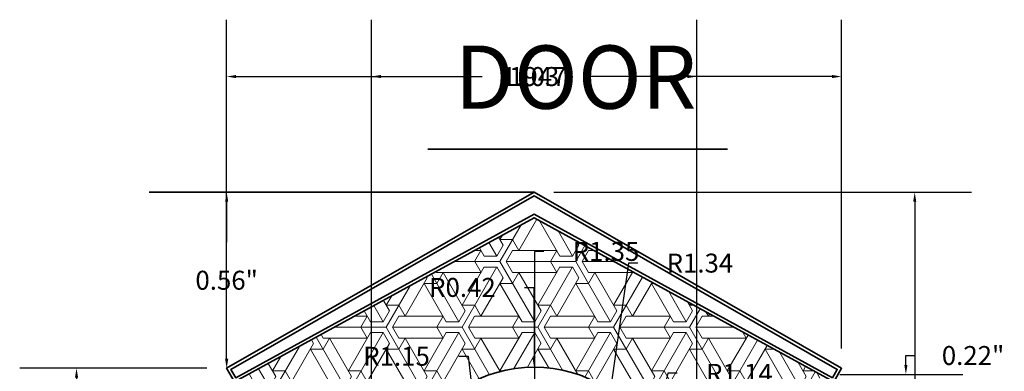
# Model space of a CAD drawing. Units: inches. Extents: x 19.36 to 24.97, y -1.46 to 4.09.
# Tile 4 of 4: x 19.36 to 22.48, y 2.98 to 4.09. Entities that reach past the tile are written whole.
import ezdxf

# ---------------------------------------------------------------- set-up
doc = ezdxf.new("R2010")
doc.units = ezdxf.units.IN
doc.header["$MEASUREMENT"] = 0
for name, color, linetype, lineweight in [('A-ANNO-DIMS', 2, 'Continuous', 18), ('A-ANNO-TEXT', 7, 'Continuous', 25), ('A-ELEV', 7, 'Continuous', 35), ('A-ELEV-PATT', 8, 'Continuous', 13)]:
    doc.layers.add(name, color=color, linetype=linetype, lineweight=lineweight)
doc.styles.get("Standard").update_dxf_attribs({"font": 'arial.ttf'})
doc.dimstyles.get("Standard").update_dxf_attribs({"dimtxt": 0.06, "dimasz": 0.03, "dimexe": 0.18, "dimexo": 0.0625, "dimgap": 0.09, "dimtad": 0, "dimtih": 1, "dimtoh": 1, "dimzin": 0, "dimdsep": 46, "dimlunit": 3, "dimtxsty": 'Standard', "dimcen": 0, "dimadec": 0, "dimazin": 0, "dimtfac": 1, "dimtofl": 0, "dimtmove": 0, "dimatfit": 3, "dimfxl": 1, "dimtolj": 1, "dimtzin": 0, "dimarcsym": 1})

# ---------------------------------------------------------------- blocks, each defined once
blk = doc.blocks.new('*D3')
at = {"layer": 'A-ANNO-DIMS', "color": 0, "lineweight": -2, "transparency": 16777216}
for p, q in [((19.9523, 3.5451), (19.8348, 3.5451)), ((20.0148, 3.5151), (20.0148, 3.3871)), ((20.0148, 3.0177), (20.0148, 3.1458)), ((19.9523, 2.9877), (19.8348, 2.9877))]:
    blk.add_line(p, q, dxfattribs=at)
at = {"layer": 'A-ANNO-DIMS', "color": 0, "transparency": 16777216}
for points in [[(20.0098, 3.5151), (20.0198, 3.5151), (20.0148, 3.5451)], [(20.0098, 3.0177), (20.0198, 3.0177), (20.0148, 2.9877)]]:
    blk.add_solid(points, dxfattribs=at)
at = {"layer": 'Defpoints', "color": 0, "transparency": 16777216}
for p in [(20.0148, 3.5451), (20.0148, 3.5451), (20.0148, 2.9877)]:
    blk.add_point(p, dxfattribs=at)
at = {"layer": 'A-ANNO-DIMS', "color": 0, "transparency": 16777216, "insert": (20.0148, 3.2664), "char_height": 0.06, "width": 0.223205, "attachment_point": 5}
blk.add_mtext('\\A1;0.56"', dxfattribs=at)
blk = doc.blocks.new('*D6')
at = {"layer": 'A-ANNO-DIMS', "color": 0, "lineweight": -2, "transparency": 16777216}
for p, q in [((22.1656, 2.9981), (22.1656, 3.0281)), ((22.1656, 3.0281), (22.1956, 3.0281)), ((21.9561, 2.9681), (22.3456, 2.9681)), ((21.9561, 2.75), (22.3456, 2.75)), ((22.1656, 2.72), (22.1656, 2.69))]:
    blk.add_line(p, q, dxfattribs=at)
at = {"layer": 'A-ANNO-DIMS', "color": 0, "transparency": 16777216}
for points in [[(22.1606, 2.9981), (22.1706, 2.9981), (22.1656, 2.9681)], [(22.1606, 2.72), (22.1706, 2.72), (22.1656, 2.75)]]:
    blk.add_solid(points, dxfattribs=at)
at = {"layer": 'Defpoints', "color": 0, "transparency": 16777216}
for p in [(21.8936, 2.9681), (22.1656, 2.9681), (21.8936, 2.75)]:
    blk.add_point(p, dxfattribs=at)
at = {"layer": 'A-ANNO-DIMS', "color": 0, "transparency": 16777216, "insert": (22.3783, 3.0281), "char_height": 0.06, "attachment_point": 5}
blk.add_mtext('\\A1;0.22"', dxfattribs=at)
blk = doc.blocks.new('*D20')
at = {"layer": 'A-ANNO-DIMS', "color": 0, "lineweight": -2, "transparency": 16777216}
for p, q in [((21.0509, 3.5451), (22.3736, 3.5451)), ((22.1936, 3.5151), (22.1936, 1.9182)), ((22.1936, 0.08), (22.1936, 1.6769)), ((22.0261, 0.05), (22.3736, 0.05))]:
    blk.add_line(p, q, dxfattribs=at)
at = {"layer": 'A-ANNO-DIMS', "color": 0, "transparency": 16777216}
for points in [[(22.1886, 3.5151), (22.1986, 3.5151), (22.1936, 3.5451)], [(22.1886, 0.08), (22.1986, 0.08), (22.1936, 0.05)]]:
    blk.add_solid(points, dxfattribs=at)
at = {"layer": 'Defpoints', "color": 0, "transparency": 16777216}
for p in [(20.9884, 3.5451), (22.1936, 3.5451), (21.9636, 0.05)]:
    blk.add_point(p, dxfattribs=at)
at = {"layer": 'A-ANNO-DIMS', "color": 0, "transparency": 16777216, "insert": (22.1936, 1.7976), "char_height": 0.06, "attachment_point": 5}
blk.add_mtext('\\A1;3.495', dxfattribs=at)
blk = doc.blocks.new('*D21')
at = {"layer": 'A-ANNO-DIMS', "color": 0, "lineweight": -2, "transparency": 16777216}
for p, q in [((20.4736, 0.1125), (20.4736, 4.0914)), ((21.5036, 0.1125), (21.5036, 4.0914)), ((20.5036, 3.9114), (20.8235, 3.9114)), ((21.4736, 3.9114), (21.1537, 3.9114))]:
    blk.add_line(p, q, dxfattribs=at)
at = {"layer": 'A-ANNO-DIMS', "color": 0, "transparency": 16777216}
for points in [[(20.5036, 3.9164), (20.5036, 3.9064), (20.4736, 3.9114)], [(21.4736, 3.9164), (21.4736, 3.9064), (21.5036, 3.9114)]]:
    blk.add_solid(points, dxfattribs=at)
at = {"layer": 'Defpoints', "color": 0, "transparency": 16777216}
for p in [(21.5036, 3.9114), (20.4736, 0.05), (21.5036, 0.05)]:
    blk.add_point(p, dxfattribs=at)
at = {"layer": 'A-ANNO-DIMS', "color": 0, "transparency": 16777216, "insert": (20.9886, 3.9114), "char_height": 0.06, "attachment_point": 5}
blk.add_mtext('\\A1;1.03', dxfattribs=at)
blk = doc.blocks.new('*D27')
at = {"layer": 'A-ANNO-DIMS', "color": 0, "lineweight": -2, "transparency": 16777216}
for p, q in [((19.9523, 2.9877), (19.3594, 2.9877)), ((19.5394, 2.9577), (19.5394, 1.6395)), ((19.5394, 0.08), (19.5394, 1.3982)), ((19.9511, 0.05), (19.3594, 0.05))]:
    blk.add_line(p, q, dxfattribs=at)
at = {"layer": 'A-ANNO-DIMS', "color": 0, "transparency": 16777216}
for points in [[(19.5344, 2.9577), (19.5444, 2.9577), (19.5394, 2.9877)], [(19.5344, 0.08), (19.5444, 0.08), (19.5394, 0.05)]]:
    blk.add_solid(points, dxfattribs=at)
at = {"layer": 'Defpoints', "color": 0, "transparency": 16777216}
for p in [(20.0148, 2.9877), (19.5394, 0.05), (20.0136, 0.05)]:
    blk.add_point(p, dxfattribs=at)
at = {"layer": 'A-ANNO-DIMS', "color": 0, "transparency": 16777216, "insert": (19.5394, 1.5189), "char_height": 0.06, "attachment_point": 5}
blk.add_mtext('\\A1;2.938', dxfattribs=at)
blk = doc.blocks.new('*D28')
at = {"layer": 'A-ANNO-DIMS', "color": 0, "lineweight": -2, "transparency": 16777216}
for p, q in [((20.0148, 3.0502), (20.0148, 4.0914)), ((21.962, 3.0502), (21.962, 4.0914)), ((20.0448, 3.9114), (20.8, 3.9114)), ((21.932, 3.9114), (21.1768, 3.9114))]:
    blk.add_line(p, q, dxfattribs=at)
at = {"layer": 'A-ANNO-DIMS', "color": 0, "transparency": 16777216}
for points in [[(20.0448, 3.9164), (20.0448, 3.9064), (20.0148, 3.9114)], [(21.932, 3.9164), (21.932, 3.9064), (21.962, 3.9114)]]:
    blk.add_solid(points, dxfattribs=at)
at = {"layer": 'Defpoints', "color": 0, "transparency": 16777216}
for p in [(21.962, 3.9114), (20.0148, 2.9877), (21.962, 2.9877)]:
    blk.add_point(p, dxfattribs=at)
at = {"layer": 'A-ANNO-DIMS', "color": 0, "transparency": 16777216, "insert": (20.9884, 3.9114), "char_height": 0.06, "attachment_point": 5}
blk.add_mtext('\\A1;1.947', dxfattribs=at)
blk = doc.blocks.new('*D36')
at = {"layer": 'A-ANNO-DIMS', "color": 0, "lineweight": -2, "transparency": 16777216}
for p, q in [((20.9578, 3.2437), (20.9878, 3.2437)), ((20.9878, 3.2437), (20.988, 3.0217))]:
    blk.add_line(p, q, dxfattribs=at)
at = {"layer": 'A-ANNO-DIMS', "color": 0, "transparency": 16777216}
blk.add_solid([(20.993, 3.0217), (20.983, 3.0217), (20.988, 2.9917)], dxfattribs=at)
at = {"layer": 'Defpoints', "color": 0, "transparency": 16777216}
for p in [(20.988, 2.9917), (20.9884, 2.5717)]:
    blk.add_point(p, dxfattribs=at)
at = {"layer": 'A-ANNO-DIMS', "color": 0, "transparency": 16777216, "insert": (20.7614, 3.2437), "char_height": 0.06, "attachment_point": 5}
blk.add_mtext('\\A1;R0.42', dxfattribs=at)
blk = doc.blocks.new('*D37')
at = {"layer": 'A-ANNO-DIMS', "color": 0, "lineweight": -2, "transparency": 16777216}
for p, q in [((20.9892, 3.3577), (20.989, 2.5805)), ((21.0192, 3.3577), (20.9892, 3.3577))]:
    blk.add_line(p, q, dxfattribs=at)
at = {"layer": 'A-ANNO-DIMS', "color": 0, "transparency": 16777216}
blk.add_solid([(20.984, 2.5806), (20.994, 2.5805), (20.989, 2.5505)], dxfattribs=at)
at = {"layer": 'Defpoints', "color": 0, "transparency": 16777216}
for p in [(20.989, 2.5505), (20.9886, 1.2054)]:
    blk.add_point(p, dxfattribs=at)
at = {"layer": 'A-ANNO-DIMS', "color": 0, "transparency": 16777216, "insert": (21.2161, 3.3577), "char_height": 0.06, "attachment_point": 5}
blk.add_mtext('\\A1;R1.35', dxfattribs=at)
blk = doc.blocks.new('*D38')
at = {"layer": 'A-ANNO-DIMS', "color": 0, "lineweight": -2, "transparency": 16777216}
for p, q in [((21.2869, 3.3207), (21.1793, 2.5572)), ((21.3169, 3.3207), (21.2869, 3.3207))]:
    blk.add_line(p, q, dxfattribs=at)
at = {"layer": 'A-ANNO-DIMS', "color": 0, "transparency": 16777216}
blk.add_solid([(21.1743, 2.5579), (21.1842, 2.5565), (21.1751, 2.5275)], dxfattribs=at)
at = {"layer": 'Defpoints', "color": 0, "transparency": 16777216}
for p in [(21.1751, 2.5275), (20.9886, 1.2054)]:
    blk.add_point(p, dxfattribs=at)
at = {"layer": 'A-ANNO-DIMS', "color": 0, "transparency": 16777216, "insert": (21.5134, 3.3207), "char_height": 0.06, "attachment_point": 5}
blk.add_mtext('\\A1;R1.34', dxfattribs=at)
blk = doc.blocks.new('*D39')
at = {"layer": 'A-ANNO-DIMS', "color": 0, "lineweight": -2, "transparency": 16777216}
for p, q in [((20.7496, 3.0257), (20.7796, 3.0257)), ((20.7796, 3.0257), (20.8546, 2.3729))]:
    blk.add_line(p, q, dxfattribs=at)
at = {"layer": 'A-ANNO-DIMS', "color": 0, "transparency": 16777216}
blk.add_solid([(20.8595, 2.3734), (20.8496, 2.3723), (20.858, 2.3431)], dxfattribs=at)
at = {"layer": 'Defpoints', "color": 0, "transparency": 16777216}
for p in [(20.858, 2.3431), (20.9886, 1.2054)]:
    blk.add_point(p, dxfattribs=at)
at = {"layer": 'A-ANNO-DIMS', "color": 0, "transparency": 16777216, "insert": (20.5527, 3.0257), "char_height": 0.06, "attachment_point": 5}
blk.add_mtext('\\A1;R1.15', dxfattribs=at)
blk = doc.blocks.new('*D40')
at = {"layer": 'A-ANNO-DIMS', "color": 0, "lineweight": -2, "transparency": 16777216}
for p, q in [((21.4117, 2.9717), (21.2601, 2.3385)), ((21.4417, 2.9717), (21.4117, 2.9717))]:
    blk.add_line(p, q, dxfattribs=at)
at = {"layer": 'A-ANNO-DIMS', "color": 0, "transparency": 16777216}
blk.add_solid([(21.2552, 2.3397), (21.2649, 2.3373), (21.2531, 2.3093)], dxfattribs=at)
at = {"layer": 'Defpoints', "color": 0, "transparency": 16777216}
for p in [(21.2531, 2.3093), (20.9886, 1.2054)]:
    blk.add_point(p, dxfattribs=at)
at = {"layer": 'A-ANNO-DIMS', "color": 0, "transparency": 16777216, "insert": (21.6383, 2.9717), "char_height": 0.06, "attachment_point": 5}
blk.add_mtext('\\A1;R1.14', dxfattribs=at)

msp = doc.modelspace()

# ---------------------------------------------------------------- hatches: boundary and pattern name
at = {"layer": 'A-ELEV-PATT'}
h = msp.add_hatch(dxfattribs=at)
h.set_pattern_fill('ESCHER', color=256, scale=0.2)
h.paths.add_polyline_path([(20.9884, 3.4642), (20.0836, 2.9685), (20.0836, 2.75), (20.1136, 2.75), (20.3136, 2.75), (20.3636, 2.75), (20.4136, 2.75), (20.6081, 2.75, -0.635528), (21.3686, 2.75), (21.5636, 2.75), (21.6136, 2.75), (21.6636, 2.75), (21.8636, 2.75), (21.8936, 2.75), (21.8936, 2.9682)])

# ---------------------------------------------------------------- linework, layer by layer
at = {"layer": 'A-ELEV'}
for p, q in [((20.6519, 3.6814), (21.6005, 3.6814)), ((20.9884, 3.5451), (19.7694, 3.5451))]:
    msp.add_line(p, q, dxfattribs=at)
for points in [[(21.937, 2.9444), (21.962, 2.9877), (20.9884, 3.5451), (20.0148, 2.9877), (20.0398, 2.9444), (20.9884, 3.4642)], [(21.9332, 2.9579), (21.9483, 2.9841), (20.9884, 3.5336), (20.0285, 2.9841), (20.0436, 2.9579), (20.9884, 3.4756)]]:
    msp.add_lwpolyline(points, close=True, dxfattribs=at)
msp.add_arc((20.9884, 2.5717), 0.42, 25.1258, 154.8742, dxfattribs=at)

# ---------------------------------------------------------------- texts
at = {"layer": 'A-ANNO-TEXT', "insert": (20.7367, 4.0095), "char_height": 0.2, "attachment_point": 1}
msp.add_mtext_dynamic_manual_height_columns('DOOR', width=0.69867, gutter_width=1, heights=[0], dxfattribs=at)

# ---------------------------------------------------------------- dimensions: what is measured, and where the dimension line sits
at = {"layer": 'A-ANNO-DIMS'}
for base, p1, p2, override, picture, middle in [((21.962, 3.9114), (20.0148, 2.9877), (21.962, 2.9877), {"dimdec": 3, "dimlfac": 1, "dimrnd": 0, "dimzin": 0, "dimdsep": 46, "dimlunit": 2}, '*D28', (20.9884, 3.9114)), ((21.5036, 3.9114), (20.4736, 0.05), (21.5036, 0.05), {"dimdec": 2, "dimlfac": 1, "dimrnd": 0, "dimzin": 0, "dimdsep": 46, "dimlunit": 2}, '*D21', (20.9886, 3.9114))]:
    dim = msp.add_linear_dim(base=base, p1=p1, p2=p2, dimstyle='Standard', override=override, dxfattribs=at)
    dim.commit()
    dim.dimension.update_dxf_attribs({"geometry": picture, "text_midpoint": middle})
for base, p1, p2, override, picture, middle in [((20.0148, 3.5451), (20.0148, 2.9877), (20.0148, 3.5451), {"dimclrd": 0, "dimclre": 0, "dimclrt": 0}, '*D3', (20.0148, 3.2664)), ((22.1936, 3.5451), (21.9636, 0.05), (20.9884, 3.5451), {"dimdec": 3, "dimlfac": 1, "dimrnd": 0, "dimzin": 0, "dimdsep": 46, "dimlunit": 2}, '*D20', (22.1936, 1.7976)), ((22.1656, 2.9681), (21.8936, 2.75), (21.8936, 2.9681), {"dimclrd": 0, "dimclre": 0, "dimclrt": 0}, '*D6', (22.3783, 3.0281)), ((19.5394, 0.05), (20.0148, 2.9877), (20.0136, 0.05), {"dimdec": 3, "dimlfac": 1, "dimrnd": 0, "dimzin": 0, "dimdsep": 46, "dimlunit": 2}, '*D27', (19.5394, 1.5189))]:
    dim = msp.add_linear_dim(base=base, p1=p1, p2=p2, angle=90, dimstyle='Standard', override=override, dxfattribs=at)
    dim.commit()
    dim.dimension.update_dxf_attribs({"geometry": picture, "text_midpoint": middle})
for center, mpoint, picture, middle in [((20.9886, 1.2054), (20.989, 2.5505), '*D37', (21.2161, 3.3577)), ((20.9886, 1.2054), (21.1751, 2.5275), '*D38', (21.5134, 3.3207)), ((20.9884, 2.5717), (20.988, 2.9917), '*D36', (20.7614, 3.2437)), ((20.9886, 1.2054), (20.858, 2.3431), '*D39', (20.5527, 3.0257)), ((20.9886, 1.2054), (21.2531, 2.3093), '*D40', (21.6383, 2.9717))]:
    dim = msp.add_radius_dim(center=center, mpoint=mpoint, dimstyle='Standard', override={"dimdec": 2, "dimlfac": 1, "dimrnd": 0, "dimzin": 0, "dimdsep": 46, "dimlunit": 2}, dxfattribs=at)
    dim.commit()
    dim.dimension.update_dxf_attribs({"geometry": picture, "text_midpoint": middle, "dimtype": 164})

doc.saveas('drawing.dxf')
